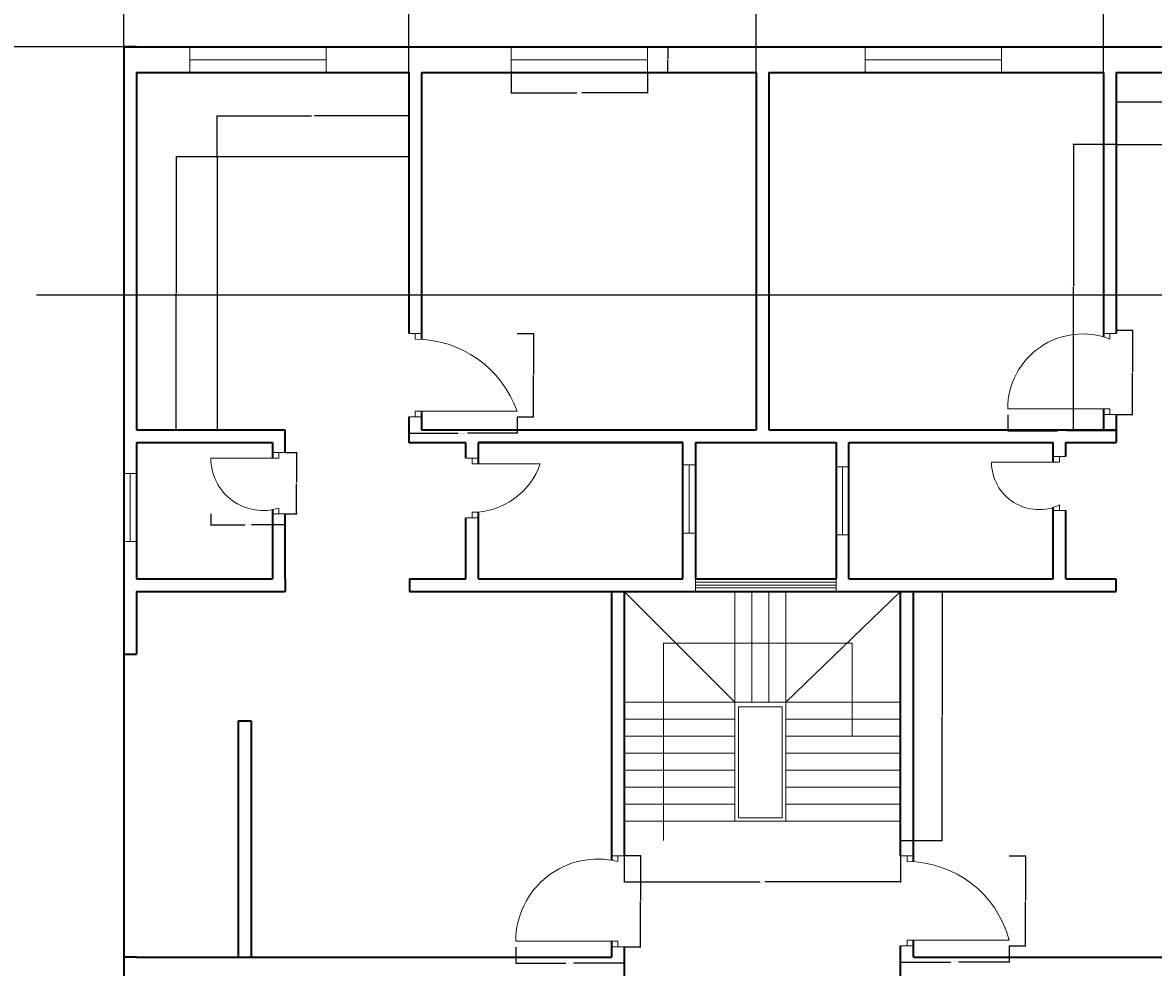
# Model space of a CAD drawing. Units: inches. Extents: x 2043 to 3387, y 1535 to 2797.
# Tile 5 of 7: x 2688 to 3087, y 2002 to 2335. Entities that reach past the tile are written whole.
import ezdxf

# ---------------------------------------------------------------- set-up
doc = ezdxf.new("R2010")
doc.units = ezdxf.units.IN
for name, color, linetype, lineweight in [('A-ANNO-DIMS', 2, 'Continuous', 18), ('A-ANNO-SYMB', 2, 'Continuous', 25), ('A-DOOR', 3, 'Continuous', 18), ('A-FLOR-FIXT', 9, 'Continuous', 25), ('A-FLOR-STRS', 2, 'Continuous', 18), ('A-GLAZ', 4, 'Continuous', 18), ('A-WALL', 7, 'Continuous', 35)]:
    doc.layers.add(name, color=color, linetype=linetype, lineweight=lineweight)
doc.styles.get("Standard").update_dxf_attribs({"font": 'arial.ttf'})
doc.dimstyles.get("Standard").update_dxf_attribs({"dimtxt": 0.18, "dimasz": 0.18, "dimexe": 0.18, "dimexo": 0.0625, "dimgap": 0.09, "dimtad": 0, "dimtih": 1, "dimtoh": 1, "dimdec": 4, "dimzin": 0, "dimdsep": 46, "dimtxsty": 'Standard', "dimcen": 0.09, "dimadec": 0, "dimazin": 0, "dimtfac": 1, "dimtdec": 4, "dimtofl": 0, "dimtmove": 0, "dimatfit": 3, "dimfxl": 1, "dimtolj": 1, "dimtzin": 0, "dimarcsym": 0})

# ---------------------------------------------------------------- blocks, each defined once
blk = doc.blocks.new('DOOR-24-WC-NW')
for p, q in [((21.75, 21.53), (26.25, 21.53)), ((26.25, 21.53), (24, 21.53)), ((24, 21.53), (24, 19.53)), ((24, 19.53), (0, 19.53)), ((24, 0), (24, 2)), ((26.25, 0), (21.75, 0)), ((21.75, 0), (24, 0))]:
    blk.add_line(p, q)
blk.add_arc((18.4, 19.53), 18.41, 180, 287.6967)
blk = doc.blocks.new('DOOR-36-BED-NW')
for p, q in [((0, 29.41), (4.5, 29.41)), ((4.5, 29.41), (2.25, 29.41)), ((2.25, 29.41), (2.25, 27.41)), ((4.5, 0), (0, 0)), ((0, 0), (2.25, 0)), ((2.25, 0), (2.25, 2)), ((2.25, 2), (38.25, 2))]:
    blk.add_line(p, q)
blk.add_arc((2.25, -10.79), 38.2, 19.5607, 90)
blk = doc.blocks.new('DOOR-36-BED-NE')
for p, q in [((33.75, 28.58), (38.25, 28.58)), ((38.25, 28.58), (36, 28.58)), ((36, 28.58), (36, 26.58)), ((36, 2), (0, 2)), ((38.25, 0), (33.75, 0)), ((33.75, 0), (36, 0)), ((36, 0), (36, 2))]:
    blk.add_line(p, q)
blk.add_arc((26.39, 2), 26.39, 68.6481, 180)
blk = doc.blocks.new('DOOR-24-BATH-NW')
for p, q in [((0, 21.1), (4.5, 21.1)), ((4.5, 21.1), (2.25, 21.1)), ((2.25, 21.1), (2.25, 19.1)), ((2.25, 19.1), (26.25, 19.1)), ((2.25, 0), (2.25, 2)), ((0, 0), (4.5, 0)), ((4.5, 0), (2.25, 0))]:
    blk.add_line(p, q)
blk.add_arc((2.25, 27.39), 25.39, 270, 340.9383)
blk = doc.blocks.new('DOOR-24-BATH-NE')
for p, q in [((24, 17.07), (0, 17.07)), ((26.25, 19.07), (21.75, 19.07)), ((21.75, 19.07), (24, 19.07)), ((24, 19.07), (24, 17.07)), ((24, 0), (24, 2)), ((21.75, 0), (26.25, 0)), ((26.25, 0), (24, 0))]:
    blk.add_line(p, q)
blk.add_arc((16.73, 17.07), 16.73, 180, 295.7467)
blk = doc.blocks.new('DOOR-36-ENTRY-NW')
for p, q in [((33.75, 32.08), (38.25, 32.08)), ((38.25, 32.08), (36, 32.08)), ((36, 32.08), (36, 30.08)), ((36, 2), (0, 2)), ((33.75, 0), (38.25, 0)), ((36, 0), (36, 2)), ((38.25, 0), (36, 0))]:
    blk.add_line(p, q)
blk.add_arc((28.95, 2), 28.95, 75.8996, 180)
blk = doc.blocks.new('DOOR-36-ENTRY-NE')
for p, q in [((0, 31.7), (3.27, 31.7)), ((4.5, 31.7), (2.28, 31.7)), ((2.28, 31.7), (2.28, 29.7)), ((3.27, 31.7), (4.5, 31.7)), ((0, 0), (4.5, 0)), ((4.5, 0), (0, 0)), ((0, 0), (2.25, 0)), ((2.25, 0), (2.25, 2)), ((2.25, 2), (38.25, 2))]:
    blk.add_line(p, q)
blk.add_arc((2.28, -7.5), 37.2, 14.7934, 90)
blk = doc.blocks.new('COUNTER-L-NW')
for p, q in [((67.52, 96.23), (0, 96.23)), ((0, 96.23), (0, 0))]:
    blk.add_line(p, q)
blk = doc.blocks.new('COUNTER-L-NE')
for p, q in [((0, 100.61), (68.19, 100.61)), ((68.19, 100.61), (68.19, 0))]:
    blk.add_line(p, q)
blk = doc.blocks.new('STAIR-U-RETURN')
for p, q in [((0, 87.81), (0, 48.81)), ((39, 48.81), (0, 87.81)), ((39, 48.81), (39, 87.81)), ((45, 48.81), (45, 87.81)), ((51, 48.81), (51, 87.81)), ((57, 48.81), (57, 87.81)), ((57, 48.81), (97.5, 87.81)), ((97.5, 87.81), (58.5, 87.81)), ((13.82, 0), (13.82, 69.54)), ((13.82, 69.54), (80.42, 69.54)), ((80.42, 69.54), (80.42, 36.81)), ((0, 48.81), (39, 48.81)), ((57, 48.81), (39, 48.81)), ((39, 48.81), (39, 48.81)), ((39, 48.81), (39, 6.81)), ((57, 48.81), (57, 6.81)), ((57, 48.81), (97.5, 48.81)), ((0, 42.81), (39, 42.81)), ((57, 42.81), (97.5, 42.81)), ((0, 36.81), (39, 36.81)), ((57, 36.81), (97.5, 36.81)), ((0, 30.81), (39, 30.81)), ((57, 30.81), (97.5, 30.81)), ((0, 24.81), (39, 24.81)), ((57, 24.81), (97.5, 24.81)), ((0, 18.81), (39, 18.81)), ((57, 18.81), (97.5, 18.81)), ((0, 12.81), (39, 12.81)), ((57, 12.81), (97.5, 12.81)), ((0, 6.81), (39, 6.81)), ((39, 6.81), (57, 6.81)), ((57, 6.81), (97.5, 6.81))]:
    blk.add_line(p, q)
blk.add_lwpolyline([(40.29, 47.17), (55.75, 47.17), (55.75, 8.03), (40.29, 8.03)], close=True)
blk = doc.blocks.new('WIN-48-PLAN')
for p, q in [((0, 9), (0, 0)), ((48, 4.5), (48, 9)), ((48, 9), (48, 0)), ((0, 0), (0, 4.5)), ((0, 4.5), (48, 4.5))]:
    blk.add_line(p, q)
blk = doc.blocks.new('WIN-48-N-JAMB')
for p, q in [((0, 9), (0, 0)), ((0, 0), (0, 9)), ((0, 9), (0, 4.5)), ((48, 4.5), (48, 9)), ((48, 9), (48, 0)), ((0, 4.5), (48, 4.5))]:
    blk.add_line(p, q)
blk = doc.blocks.new('VENT-24-W')
for p, q in [((0, 24), (4.5, 24)), ((4.5, 24), (0, 24)), ((0, 24), (0, 0)), ((2.25, 24), (2.25, 0)), ((0, 0), (4.5, 0))]:
    blk.add_line(p, q)
blk = doc.blocks.new('VENT-24-PLAN')
for p, q in [((0, 24), (4.5, 24)), ((4.5, 24), (2.25, 24)), ((2.25, 24), (2.25, 0)), ((2.25, 0), (0, 0)), ((0, 0), (4.5, 0))]:
    blk.add_line(p, q)
blk = doc.blocks.new('WIN-STAIR-DUCT')
for p, q in [((0, 4.5), (0, 0)), ((49.62, 4.5), (49.62, 0)), ((0, 2.25), (0, 3.25)), ((0, 3.25), (49.62, 3.25)), ((49.62, 2.25), (0, 2.25)), ((49.62, 1.25), (0, 1.25)), ((49.62, 3.25), (49.62, 2.25)), ((49.62, 2.25), (49.62, 2.25)), ((49.62, 2.25), (49.62, 1.25))]:
    blk.add_line(p, q)
blk = doc.blocks.new('*D41')
at = {"layer": 'A-ANNO-DIMS', "color": 0, "lineweight": -2, "transparency": 16777216}
for p, q in [((2860.38, 2317.31), (2860.38, 2310)), ((2908.38, 2317.31), (2908.38, 2310)), ((2860.56, 2310.18), (2883.48, 2310.18)), ((2908.2, 2310.18), (2885.28, 2310.18))]:
    blk.add_line(p, q, dxfattribs=at)
at = {"layer": 'A-ANNO-DIMS', "color": 0, "transparency": 16777216}
for points in [[(2860.56, 2310.21), (2860.56, 2310.15), (2860.38, 2310.18)], [(2908.2, 2310.21), (2908.2, 2310.15), (2908.38, 2310.18)]]:
    blk.add_solid(points, dxfattribs=at)
at = {"layer": 'Defpoints', "color": 0, "transparency": 16777216}
for p in [(2860.38, 2317.38), (2908.38, 2317.38), (2908.38, 2310.18)]:
    blk.add_point(p, dxfattribs=at)
at = {"layer": 'A-ANNO-DIMS', "color": 0, "transparency": 16777216, "insert": (2884.38, 2310.18), "char_height": 0.18, "attachment_point": 5}
blk.add_mtext('\\A1;JAMB 48 TYP.', dxfattribs=at)
blk = doc.blocks.new('*D42')
at = {"layer": 'A-ANNO-DIMS', "color": 0, "lineweight": -2, "transparency": 16777216}
for p, q in [((2908.45, 2326.38), (2915.76, 2326.38)), ((2915.58, 2326.2), (2915.58, 2322.06)), ((2915.58, 2317.56), (2915.58, 2321.7)), ((2908.45, 2317.38), (2915.76, 2317.38))]:
    blk.add_line(p, q, dxfattribs=at)
at = {"layer": 'A-ANNO-DIMS', "color": 0, "transparency": 16777216}
for points in [[(2915.55, 2326.2), (2915.61, 2326.2), (2915.58, 2326.38)], [(2915.55, 2317.56), (2915.61, 2317.56), (2915.58, 2317.38)]]:
    blk.add_solid(points, dxfattribs=at)
at = {"layer": 'Defpoints', "color": 0, "transparency": 16777216}
for p in [(2908.38, 2326.38), (2915.58, 2326.38), (2908.38, 2317.38)]:
    blk.add_point(p, dxfattribs=at)
at = {"layer": 'A-ANNO-DIMS', "color": 0, "transparency": 16777216, "insert": (2915.58, 2321.88), "char_height": 0.18, "attachment_point": 5}
blk.add_mtext('\\A1;9 TYP.', dxfattribs=at)
blk = doc.blocks.new('*D49')
at = {"layer": 'A-ANNO-DIMS', "color": 0, "lineweight": -2, "transparency": 16777216}
for p, q in [((2754.46, 2161.73), (2754.46, 2157.68)), ((2780.71, 2161.73), (2780.71, 2157.68)), ((2754.64, 2157.86), (2766.4, 2157.86)), ((2780.53, 2157.86), (2768.77, 2157.86))]:
    blk.add_line(p, q, dxfattribs=at)
at = {"layer": 'A-ANNO-DIMS', "color": 0, "transparency": 16777216}
for points in [[(2754.64, 2157.89), (2754.64, 2157.83), (2754.46, 2157.86)], [(2780.53, 2157.89), (2780.53, 2157.83), (2780.71, 2157.86)]]:
    blk.add_solid(points, dxfattribs=at)
at = {"layer": 'Defpoints', "color": 0, "transparency": 16777216}
for p in [(2754.46, 2161.79), (2780.71, 2161.79), (2780.71, 2157.86)]:
    blk.add_point(p, dxfattribs=at)
at = {"layer": 'A-ANNO-DIMS', "color": 0, "transparency": 16777216, "insert": (2767.58, 2157.86), "char_height": 0.18, "attachment_point": 5}
blk.add_mtext('\\A1;WC DOOR 26 TYP.', dxfattribs=at)
blk = doc.blocks.new('*D50')
at = {"layer": 'A-ANNO-DIMS', "color": 0, "lineweight": -2, "transparency": 16777216}
for p, q in [((2780.77, 2183.33), (2784.83, 2183.33)), ((2784.65, 2183.15), (2784.65, 2172.74)), ((2784.65, 2161.97), (2784.65, 2172.38)), ((2780.77, 2161.79), (2784.83, 2161.79))]:
    blk.add_line(p, q, dxfattribs=at)
at = {"layer": 'A-ANNO-DIMS', "color": 0, "transparency": 16777216}
for points in [[(2784.62, 2183.15), (2784.68, 2183.15), (2784.65, 2183.33)], [(2784.62, 2161.97), (2784.68, 2161.97), (2784.65, 2161.79)]]:
    blk.add_solid(points, dxfattribs=at)
at = {"layer": 'Defpoints', "color": 0, "transparency": 16777216}
for p in [(2780.71, 2183.33), (2784.65, 2183.33), (2780.71, 2161.79)]:
    blk.add_point(p, dxfattribs=at)
at = {"layer": 'A-ANNO-DIMS', "color": 0, "transparency": 16777216, "insert": (2784.65, 2172.56), "char_height": 0.18, "attachment_point": 5}
blk.add_mtext('\\A1;22 TYP.', dxfattribs=at)
blk = doc.blocks.new('*D65')
at = {"layer": 'A-ANNO-DIMS', "color": 0, "lineweight": -2, "transparency": 16777216}
for p, q in [((2861.96, 2008.98), (2861.96, 2003.13)), ((2900.21, 2008.98), (2900.21, 2003.13)), ((2862.14, 2003.31), (2879.69, 2003.31)), ((2900.03, 2003.31), (2882.48, 2003.31))]:
    blk.add_line(p, q, dxfattribs=at)
at = {"layer": 'A-ANNO-DIMS', "color": 0, "transparency": 16777216}
for points in [[(2862.14, 2003.34), (2862.14, 2003.28), (2861.96, 2003.31)], [(2900.03, 2003.34), (2900.03, 2003.28), (2900.21, 2003.31)]]:
    blk.add_solid(points, dxfattribs=at)
at = {"layer": 'Defpoints', "color": 0, "transparency": 16777216}
for p in [(2861.96, 2009.05), (2900.21, 2009.05), (2900.21, 2003.31)]:
    blk.add_point(p, dxfattribs=at)
at = {"layer": 'A-ANNO-DIMS', "color": 0, "transparency": 16777216, "insert": (2881.08, 2003.31), "char_height": 0.18, "attachment_point": 5}
blk.add_mtext('\\A1;ENTRY DOOR 38 TYP.', dxfattribs=at)
blk = doc.blocks.new('*D66')
at = {"layer": 'A-ANNO-DIMS', "color": 0, "lineweight": -2, "transparency": 16777216}
for p, q in [((2900.27, 2041.29), (2906.13, 2041.29)), ((2905.95, 2041.11), (2905.95, 2025.35)), ((2905.95, 2009.23), (2905.95, 2024.99)), ((2900.27, 2009.05), (2906.13, 2009.05))]:
    blk.add_line(p, q, dxfattribs=at)
at = {"layer": 'A-ANNO-DIMS', "color": 0, "transparency": 16777216}
for points in [[(2905.92, 2041.11), (2905.98, 2041.11), (2905.95, 2041.29)], [(2905.92, 2009.23), (2905.98, 2009.23), (2905.95, 2009.05)]]:
    blk.add_solid(points, dxfattribs=at)
at = {"layer": 'Defpoints', "color": 0, "transparency": 16777216}
for p in [(2900.21, 2041.29), (2905.95, 2041.29), (2900.21, 2009.05)]:
    blk.add_point(p, dxfattribs=at)
at = {"layer": 'A-ANNO-DIMS', "color": 0, "transparency": 16777216, "insert": (2905.95, 2025.17), "char_height": 0.18, "attachment_point": 5}
blk.add_mtext('\\A1;32 TYP.', dxfattribs=at)
blk = doc.blocks.new('*D67')
at = {"layer": 'A-ANNO-DIMS', "color": 0, "lineweight": -2, "transparency": 16777216}
for p, q in [((2997.71, 2009.36), (2997.71, 2003.5)), ((3035.96, 2009.36), (3035.96, 2003.5)), ((2997.89, 2003.68), (3015.44, 2003.68)), ((3035.78, 2003.68), (3018.23, 2003.68))]:
    blk.add_line(p, q, dxfattribs=at)
at = {"layer": 'A-ANNO-DIMS', "color": 0, "transparency": 16777216}
for points in [[(2997.89, 2003.71), (2997.89, 2003.65), (2997.71, 2003.68)], [(3035.78, 2003.71), (3035.78, 2003.65), (3035.96, 2003.68)]]:
    blk.add_solid(points, dxfattribs=at)
at = {"layer": 'Defpoints', "color": 0, "transparency": 16777216}
for p in [(2997.71, 2009.42), (3035.96, 2009.42), (3035.96, 2003.68)]:
    blk.add_point(p, dxfattribs=at)
at = {"layer": 'A-ANNO-DIMS', "color": 0, "transparency": 16777216, "insert": (3016.83, 2003.68), "char_height": 0.18, "attachment_point": 5}
blk.add_mtext('\\A1;ENTRY DOOR 38 TYP.', dxfattribs=at)
blk = doc.blocks.new('*D68')
at = {"layer": 'A-ANNO-DIMS', "color": 0, "lineweight": -2, "transparency": 16777216}
for p, q in [((3036.02, 2041.12), (3041.88, 2041.12)), ((3041.7, 2040.94), (3041.7, 2025.45)), ((3041.7, 2009.6), (3041.7, 2025.09)), ((3036.02, 2009.42), (3041.88, 2009.42))]:
    blk.add_line(p, q, dxfattribs=at)
at = {"layer": 'A-ANNO-DIMS', "color": 0, "transparency": 16777216}
for points in [[(3041.67, 2040.94), (3041.73, 2040.94), (3041.7, 2041.12)], [(3041.67, 2009.6), (3041.73, 2009.6), (3041.7, 2009.42)]]:
    blk.add_solid(points, dxfattribs=at)
at = {"layer": 'Defpoints', "color": 0, "transparency": 16777216}
for p in [(3035.96, 2041.12), (3041.7, 2041.12), (3035.96, 2009.42)]:
    blk.add_point(p, dxfattribs=at)
at = {"layer": 'A-ANNO-DIMS', "color": 0, "transparency": 16777216, "insert": (3041.7, 2025.27), "char_height": 0.18, "attachment_point": 5}
blk.add_mtext('\\A1;32 TYP.', dxfattribs=at)
blk = doc.blocks.new('*D73')
at = {"layer": 'A-ANNO-DIMS', "color": 0, "lineweight": -2, "transparency": 16777216}
for p, q in [((2824.21, 2195.88), (2824.21, 2190.03)), ((2862.46, 2195.88), (2862.46, 2190.03)), ((2824.39, 2190.21), (2841.71, 2190.21)), ((2862.28, 2190.21), (2844.95, 2190.21))]:
    blk.add_line(p, q, dxfattribs=at)
at = {"layer": 'A-ANNO-DIMS', "color": 0, "transparency": 16777216}
for points in [[(2824.39, 2190.24), (2824.39, 2190.18), (2824.21, 2190.21)], [(2862.28, 2190.24), (2862.28, 2190.18), (2862.46, 2190.21)]]:
    blk.add_solid(points, dxfattribs=at)
at = {"layer": 'Defpoints', "color": 0, "transparency": 16777216}
for p in [(2824.21, 2195.94), (2862.46, 2195.94), (2862.46, 2190.21)]:
    blk.add_point(p, dxfattribs=at)
at = {"layer": 'A-ANNO-DIMS', "color": 0, "transparency": 16777216, "insert": (2843.33, 2190.21), "char_height": 0.18, "attachment_point": 5}
blk.add_mtext('\\A1;BEDROOM DOOR 38 TYP.', dxfattribs=at)
blk = doc.blocks.new('*D74')
at = {"layer": 'A-ANNO-DIMS', "color": 0, "lineweight": -2, "transparency": 16777216}
for p, q in [((2862.52, 2225.36), (2868.38, 2225.36)), ((2868.2, 2225.18), (2868.2, 2210.83)), ((2868.2, 2196.12), (2868.2, 2210.47)), ((2862.52, 2195.94), (2868.38, 2195.94))]:
    blk.add_line(p, q, dxfattribs=at)
at = {"layer": 'A-ANNO-DIMS', "color": 0, "transparency": 16777216}
for points in [[(2868.17, 2225.18), (2868.23, 2225.18), (2868.2, 2225.36)], [(2868.17, 2196.12), (2868.23, 2196.12), (2868.2, 2195.94)]]:
    blk.add_solid(points, dxfattribs=at)
at = {"layer": 'Defpoints', "color": 0, "transparency": 16777216}
for p in [(2862.46, 2225.36), (2868.2, 2225.36), (2862.46, 2195.94)]:
    blk.add_point(p, dxfattribs=at)
at = {"layer": 'A-ANNO-DIMS', "color": 0, "transparency": 16777216, "insert": (2868.2, 2210.65), "char_height": 0.18, "attachment_point": 5}
blk.add_mtext('\\A1;29 TYP.', dxfattribs=at)
blk = doc.blocks.new('*D75')
at = {"layer": 'A-ANNO-DIMS', "color": 0, "lineweight": -2, "transparency": 16777216}
for p, q in [((3035.46, 2196.71), (3035.46, 2190.86)), ((3073.71, 2196.71), (3073.71, 2190.86)), ((3035.64, 2191.04), (3052.96, 2191.04)), ((3073.53, 2191.04), (3056.2, 2191.04))]:
    blk.add_line(p, q, dxfattribs=at)
at = {"layer": 'A-ANNO-DIMS', "color": 0, "transparency": 16777216}
for points in [[(3035.64, 2191.07), (3035.64, 2191.01), (3035.46, 2191.04)], [(3073.53, 2191.07), (3073.53, 2191.01), (3073.71, 2191.04)]]:
    blk.add_solid(points, dxfattribs=at)
at = {"layer": 'Defpoints', "color": 0, "transparency": 16777216}
for p in [(3035.46, 2196.78), (3073.71, 2196.78), (3073.71, 2191.04)]:
    blk.add_point(p, dxfattribs=at)
at = {"layer": 'A-ANNO-DIMS', "color": 0, "transparency": 16777216, "insert": (3054.58, 2191.04), "char_height": 0.18, "attachment_point": 5}
blk.add_mtext('\\A1;BEDROOM DOOR 38 TYP.', dxfattribs=at)
blk = doc.blocks.new('*D76')
at = {"layer": 'A-ANNO-DIMS', "color": 0, "lineweight": -2, "transparency": 16777216}
for p, q in [((3073.77, 2226.53), (3079.63, 2226.53)), ((3079.45, 2226.35), (3079.45, 2211.84)), ((3079.45, 2196.96), (3079.45, 2211.47)), ((3073.77, 2196.78), (3079.63, 2196.78))]:
    blk.add_line(p, q, dxfattribs=at)
at = {"layer": 'A-ANNO-DIMS', "color": 0, "transparency": 16777216}
for points in [[(3079.42, 2226.35), (3079.48, 2226.35), (3079.45, 2226.53)], [(3079.42, 2196.96), (3079.48, 2196.96), (3079.45, 2196.78)]]:
    blk.add_solid(points, dxfattribs=at)
at = {"layer": 'Defpoints', "color": 0, "transparency": 16777216}
for p in [(3073.71, 2226.53), (3079.45, 2226.53), (3073.71, 2196.78)]:
    blk.add_point(p, dxfattribs=at)
at = {"layer": 'A-ANNO-DIMS', "color": 0, "transparency": 16777216, "insert": (3079.45, 2211.65), "char_height": 0.18, "attachment_point": 5}
blk.add_mtext('\\A1;30 TYP.', dxfattribs=at)
blk = doc.blocks.new('*D81')
at = {"layer": 'A-ANNO-DIMS', "color": 0, "lineweight": -2, "transparency": 16777216}
for p, q in [((2756.63, 2287.61), (2742.08, 2287.61)), ((2742.26, 2287.43), (2742.26, 2239.68)), ((2742.26, 2191.56), (2742.26, 2239.31)), ((2756.63, 2191.38), (2742.08, 2191.38))]:
    blk.add_line(p, q, dxfattribs=at)
at = {"layer": 'A-ANNO-DIMS', "color": 0, "transparency": 16777216}
for points in [[(2742.23, 2287.43), (2742.29, 2287.43), (2742.26, 2287.61)], [(2742.23, 2191.56), (2742.29, 2191.56), (2742.26, 2191.38)]]:
    blk.add_solid(points, dxfattribs=at)
at = {"layer": 'Defpoints', "color": 0, "transparency": 16777216}
for p in [(2742.26, 2287.61), (2756.69, 2287.61), (2756.69, 2191.38)]:
    blk.add_point(p, dxfattribs=at)
at = {"layer": 'A-ANNO-DIMS', "color": 0, "transparency": 16777216, "insert": (2742.26, 2239.49), "char_height": 0.18, "attachment_point": 5}
blk.add_mtext('\\A1;COUNTER 96 TYP.', dxfattribs=at)
blk = doc.blocks.new('*D82')
at = {"layer": 'A-ANNO-DIMS', "color": 0, "lineweight": -2, "transparency": 16777216}
for p, q in [((2756.69, 2287.67), (2756.69, 2302.22)), ((2756.87, 2302.04), (2789.92, 2302.04)), ((2824.03, 2302.04), (2790.98, 2302.04)), ((2824.21, 2287.67), (2824.21, 2302.22))]:
    blk.add_line(p, q, dxfattribs=at)
at = {"layer": 'A-ANNO-DIMS', "color": 0, "transparency": 16777216}
for points in [[(2756.87, 2302.07), (2756.87, 2302.01), (2756.69, 2302.04)], [(2824.03, 2302.07), (2824.03, 2302.01), (2824.21, 2302.04)]]:
    blk.add_solid(points, dxfattribs=at)
at = {"layer": 'Defpoints', "color": 0, "transparency": 16777216}
for p in [(2824.21, 2302.04), (2756.69, 2287.61), (2824.21, 2287.61)]:
    blk.add_point(p, dxfattribs=at)
at = {"layer": 'A-ANNO-DIMS', "color": 0, "transparency": 16777216, "insert": (2790.45, 2302.04), "char_height": 0.18, "attachment_point": 5}
blk.add_mtext('\\A1;68 TYP.', dxfattribs=at)
blk = doc.blocks.new('*D83')
at = {"layer": 'A-ANNO-DIMS', "color": 0, "lineweight": -2, "transparency": 16777216}
for p, q in [((3073.65, 2291.99), (3058.44, 2291.99)), ((3058.62, 2291.81), (3058.62, 2241.87)), ((3058.62, 2191.56), (3058.62, 2241.5)), ((3073.65, 2191.38), (3058.44, 2191.38))]:
    blk.add_line(p, q, dxfattribs=at)
at = {"layer": 'A-ANNO-DIMS', "color": 0, "transparency": 16777216}
for points in [[(3058.59, 2291.81), (3058.65, 2291.81), (3058.62, 2291.99)], [(3058.59, 2191.56), (3058.65, 2191.56), (3058.62, 2191.38)]]:
    blk.add_solid(points, dxfattribs=at)
at = {"layer": 'Defpoints', "color": 0, "transparency": 16777216}
for p in [(3058.62, 2291.99), (3073.71, 2291.99), (3073.71, 2191.38)]:
    blk.add_point(p, dxfattribs=at)
at = {"layer": 'A-ANNO-DIMS', "color": 0, "transparency": 16777216, "insert": (3058.62, 2241.68), "char_height": 0.18, "attachment_point": 5}
blk.add_mtext('\\A1;COUNTER 101 TYP.', dxfattribs=at)
blk = doc.blocks.new('*D84')
at = {"layer": 'A-ANNO-DIMS', "color": 0, "lineweight": -2, "transparency": 16777216}
for p, q in [((3073.71, 2292.05), (3073.71, 2307.26)), ((3073.89, 2307.08), (3107.27, 2307.08)), ((3141.72, 2307.08), (3108.33, 2307.08)), ((3141.9, 2292.05), (3141.9, 2307.26))]:
    blk.add_line(p, q, dxfattribs=at)
at = {"layer": 'A-ANNO-DIMS', "color": 0, "transparency": 16777216}
for points in [[(3073.89, 2307.11), (3073.89, 2307.05), (3073.71, 2307.08)], [(3141.72, 2307.11), (3141.72, 2307.05), (3141.9, 2307.08)]]:
    blk.add_solid(points, dxfattribs=at)
at = {"layer": 'Defpoints', "color": 0, "transparency": 16777216}
for p in [(3141.9, 2307.08), (3073.71, 2291.99), (3141.9, 2291.99)]:
    blk.add_point(p, dxfattribs=at)
at = {"layer": 'A-ANNO-DIMS', "color": 0, "transparency": 16777216, "insert": (3107.8, 2307.08), "char_height": 0.18, "attachment_point": 5}
blk.add_mtext('\\A1;68 TYP.', dxfattribs=at)
blk = doc.blocks.new('*D89')
at = {"layer": 'A-ANNO-DIMS', "color": 0, "lineweight": -2, "transparency": 16777216}
for p, q in [((2900.21, 2046.51), (2900.21, 2031.76)), ((2997.71, 2046.51), (2997.71, 2031.76)), ((2900.39, 2031.94), (2948.03, 2031.94)), ((2997.53, 2031.94), (2949.89, 2031.94))]:
    blk.add_line(p, q, dxfattribs=at)
at = {"layer": 'A-ANNO-DIMS', "color": 0, "transparency": 16777216}
for points in [[(2900.39, 2031.97), (2900.39, 2031.91), (2900.21, 2031.94)], [(2997.53, 2031.97), (2997.53, 2031.91), (2997.71, 2031.94)]]:
    blk.add_solid(points, dxfattribs=at)
at = {"layer": 'Defpoints', "color": 0, "transparency": 16777216}
for p in [(2900.21, 2046.57), (2997.71, 2046.57), (2997.71, 2031.94)]:
    blk.add_point(p, dxfattribs=at)
at = {"layer": 'A-ANNO-DIMS', "color": 0, "transparency": 16777216, "insert": (2948.96, 2031.94), "char_height": 0.18, "attachment_point": 5}
blk.add_mtext('\\A1;STAIR 98 TYP.', dxfattribs=at)
blk = doc.blocks.new('*D90')
at = {"layer": 'A-ANNO-DIMS', "color": 0, "lineweight": -2, "transparency": 16777216}
for p, q in [((2997.77, 2134.38), (3012.51, 2134.38)), ((3012.33, 2134.2), (3012.33, 2090.65)), ((3012.33, 2046.75), (3012.33, 2090.29)), ((2997.77, 2046.57), (3012.51, 2046.57))]:
    blk.add_line(p, q, dxfattribs=at)
at = {"layer": 'A-ANNO-DIMS', "color": 0, "transparency": 16777216}
for points in [[(3012.3, 2134.2), (3012.36, 2134.2), (3012.33, 2134.38)], [(3012.3, 2046.75), (3012.36, 2046.75), (3012.33, 2046.57)]]:
    blk.add_solid(points, dxfattribs=at)
at = {"layer": 'Defpoints', "color": 0, "transparency": 16777216}
for p in [(2997.71, 2134.38), (3012.33, 2134.38), (2997.71, 2046.57)]:
    blk.add_point(p, dxfattribs=at)
at = {"layer": 'A-ANNO-DIMS', "color": 0, "transparency": 16777216, "insert": (3012.33, 2090.47), "char_height": 0.18, "attachment_point": 5}
blk.add_mtext('\\A1;88 TYP.', dxfattribs=at)
blk = doc.blocks.new('*D106')
at = {"layer": 'A-ANNO-DIMS', "color": 0, "lineweight": -2, "transparency": 16777216}
for p, q in [((2723.65, 2326.38), (2660.13, 2326.38)), ((2660.31, 2326.2), (2660.31, 2006.31)), ((2660.31, 1686.06), (2660.31, 2005.95)), ((2723.65, 1685.88), (2660.13, 1685.88))]:
    blk.add_line(p, q, dxfattribs=at)
at = {"layer": 'A-ANNO-DIMS', "color": 0, "transparency": 16777216}
for points in [[(2660.28, 2326.2), (2660.34, 2326.2), (2660.31, 2326.38)], [(2660.28, 1686.06), (2660.34, 1686.06), (2660.31, 1685.88)]]:
    blk.add_solid(points, dxfattribs=at)
at = {"layer": 'Defpoints', "color": 0, "transparency": 16777216}
for p in [(2660.31, 2326.38), (2723.71, 2326.38), (2723.71, 1685.88)]:
    blk.add_point(p, dxfattribs=at)
at = {"layer": 'A-ANNO-DIMS', "color": 0, "transparency": 16777216, "insert": (2660.31, 2006.13), "char_height": 0.18, "attachment_point": 5}
blk.add_mtext('\\A1;640.5', dxfattribs=at)
blk = doc.blocks.new('*D107')
at = {"layer": 'A-ANNO-DIMS', "color": 0, "lineweight": -2, "transparency": 16777216}
for p, q in [((2723.71, 2326.44), (2723.71, 2359.26)), ((2723.89, 2359.08), (2773.57, 2359.08)), ((2824.03, 2359.08), (2774.34, 2359.08)), ((2824.21, 2317.44), (2824.21, 2359.26))]:
    blk.add_line(p, q, dxfattribs=at)
at = {"layer": 'A-ANNO-DIMS', "color": 0, "transparency": 16777216}
for points in [[(2723.89, 2359.11), (2723.89, 2359.05), (2723.71, 2359.08)], [(2824.03, 2359.11), (2824.03, 2359.05), (2824.21, 2359.08)]]:
    blk.add_solid(points, dxfattribs=at)
at = {"layer": 'Defpoints', "color": 0, "transparency": 16777216}
for p in [(2824.21, 2359.08), (2723.71, 2326.38), (2824.21, 2317.38)]:
    blk.add_point(p, dxfattribs=at)
at = {"layer": 'A-ANNO-DIMS', "color": 0, "transparency": 16777216, "insert": (2773.96, 2359.08), "char_height": 0.18, "attachment_point": 5}
blk.add_mtext('\\A1;100.5', dxfattribs=at)
blk = doc.blocks.new('*D108')
at = {"layer": 'A-ANNO-DIMS', "color": 0, "lineweight": -2, "transparency": 16777216}
for p, q in [((2824.21, 2317.44), (2824.21, 2359.26)), ((2824.39, 2359.08), (2885.07, 2359.08)), ((2946.53, 2359.08), (2885.84, 2359.08)), ((2946.71, 2317.44), (2946.71, 2359.26))]:
    blk.add_line(p, q, dxfattribs=at)
at = {"layer": 'A-ANNO-DIMS', "color": 0, "transparency": 16777216}
for points in [[(2824.39, 2359.11), (2824.39, 2359.05), (2824.21, 2359.08)], [(2946.53, 2359.11), (2946.53, 2359.05), (2946.71, 2359.08)]]:
    blk.add_solid(points, dxfattribs=at)
at = {"layer": 'Defpoints', "color": 0, "transparency": 16777216}
for p in [(2946.71, 2359.08), (2824.21, 2317.38), (2946.71, 2317.38)]:
    blk.add_point(p, dxfattribs=at)
at = {"layer": 'A-ANNO-DIMS', "color": 0, "transparency": 16777216, "insert": (2885.46, 2359.08), "char_height": 0.18, "attachment_point": 5}
blk.add_mtext('\\A1;122.5', dxfattribs=at)
blk = doc.blocks.new('*D109')
at = {"layer": 'A-ANNO-DIMS', "color": 0, "lineweight": -2, "transparency": 16777216}
for p, q in [((2946.71, 2317.44), (2946.71, 2359.26)), ((2946.89, 2359.08), (3007.57, 2359.08)), ((3069.03, 2359.08), (3008.34, 2359.08)), ((3069.21, 2317.44), (3069.21, 2359.26))]:
    blk.add_line(p, q, dxfattribs=at)
at = {"layer": 'A-ANNO-DIMS', "color": 0, "transparency": 16777216}
for points in [[(2946.89, 2359.11), (2946.89, 2359.05), (2946.71, 2359.08)], [(3069.03, 2359.11), (3069.03, 2359.05), (3069.21, 2359.08)]]:
    blk.add_solid(points, dxfattribs=at)
at = {"layer": 'Defpoints', "color": 0, "transparency": 16777216}
for p in [(3069.21, 2359.08), (2946.71, 2317.38), (3069.21, 2317.38)]:
    blk.add_point(p, dxfattribs=at)
at = {"layer": 'A-ANNO-DIMS', "color": 0, "transparency": 16777216, "insert": (3007.96, 2359.08), "char_height": 0.18, "attachment_point": 5}
blk.add_mtext('\\A1;122.5', dxfattribs=at)
blk = doc.blocks.new('*D110')
at = {"layer": 'A-ANNO-DIMS', "color": 0, "lineweight": -2, "transparency": 16777216}
for p, q in [((3069.21, 2317.44), (3069.21, 2359.26)), ((3069.39, 2359.08), (3121.43, 2359.08)), ((3174.03, 2359.08), (3121.99, 2359.08)), ((3174.21, 2326.44), (3174.21, 2359.26))]:
    blk.add_line(p, q, dxfattribs=at)
at = {"layer": 'A-ANNO-DIMS', "color": 0, "transparency": 16777216}
for points in [[(3069.39, 2359.11), (3069.39, 2359.05), (3069.21, 2359.08)], [(3174.03, 2359.11), (3174.03, 2359.05), (3174.21, 2359.08)]]:
    blk.add_solid(points, dxfattribs=at)
at = {"layer": 'Defpoints', "color": 0, "transparency": 16777216}
for p in [(3174.21, 2359.08), (3174.21, 2326.38), (3069.21, 2317.38)]:
    blk.add_point(p, dxfattribs=at)
at = {"layer": 'A-ANNO-DIMS', "color": 0, "transparency": 16777216, "insert": (3121.71, 2359.08), "char_height": 0.18, "attachment_point": 5}
blk.add_mtext('\\A1;105', dxfattribs=at)

msp = doc.modelspace()

# ---------------------------------------------------------------- linework, layer by layer
at = {"layer": 'A-ANNO-SYMB'}
msp.add_line((2693.0063, 2238.9239), (3223.9712, 2238.9239), dxfattribs=at)
at = {"layer": 'A-WALL'}
for p, q in [((2723.7086, 2326.3769), (3174.2086, 2326.3769)), ((2728.2086, 2326.3769), (2723.7086, 2326.3769)), ((2723.7086, 2326.3769), (2723.7086, 1734.4589)), ((2728.2086, 2317.3769), (2824.2086, 2317.3769)), ((2728.2086, 2317.3769), (2728.2086, 2191.3769)), ((2824.2086, 2317.3769), (2824.2086, 2225.357)), ((2828.7086, 2317.3769), (2946.7086, 2317.3769)), ((2828.7086, 2317.3769), (2828.7086, 2223.2907)), ((2946.7086, 2317.3769), (2946.7086, 2191.3769)), ((2951.2086, 2317.3769), (3069.2086, 2317.3769)), ((2951.2086, 2317.3769), (2951.2086, 2191.3769)), ((3069.2086, 2317.3769), (3069.2086, 2224.1217)), ((3073.7086, 2317.3769), (3169.7086, 2317.3769)), ((3073.7086, 2317.3769), (3073.7086, 2225.357)), ((2828.7086, 2197.9433), (2828.7086, 2191.3769)), ((3069.2086, 2198.7773), (3069.2086, 2191.3769)), ((2824.2086, 2195.9433), (2824.2086, 2186.8769)), ((3073.7086, 2196.7773), (3073.7086, 2186.8769)), ((2728.2086, 2191.3769), (2780.7086, 2191.3769)), ((2780.7086, 2183.3291), (2780.7086, 2191.3769)), ((2828.7086, 2191.3769), (2946.7086, 2191.3769)), ((2951.2086, 2191.3769), (3069.2086, 2191.3769)), ((2728.2086, 2186.8769), (2776.2086, 2186.8769)), ((2728.2086, 2186.8769), (2728.2086, 2138.8769)), ((2728.2086, 2186.8769), (2776.2086, 2186.8769)), ((2776.2086, 2186.8769), (2776.2086, 2181.3291)), ((2824.2086, 2186.8769), (2844.3641, 2186.8769)), ((2824.2086, 2186.8769), (2844.3641, 2186.8769)), ((2844.3641, 2181.3932), (2844.3641, 2186.8769)), ((2848.8641, 2186.8769), (2920.8641, 2186.8769)), ((2848.8641, 2186.8769), (2896.2086, 2186.8769)), ((2848.8641, 2179.3932), (2848.8641, 2186.8769)), ((2920.8641, 2186.8769), (2848.8641, 2186.8769)), ((2920.8641, 2138.8769), (2920.8641, 2186.8769)), ((2925.3641, 2186.8769), (2974.9865, 2186.8769)), ((2925.3641, 2186.8769), (2925.3641, 2138.8769)), ((2974.9865, 2186.8769), (2974.9865, 2138.8769)), ((2979.4865, 2186.8769), (3051.4865, 2186.8769)), ((2979.4865, 2138.8769), (2979.4865, 2186.8769)), ((3051.4865, 2179.9477), (3051.4865, 2186.8769)), ((3055.9865, 2186.8769), (3073.7086, 2186.8769)), ((3055.9865, 2181.9477), (3055.9865, 2186.8769)), ((2776.2086, 2163.2304), (2776.2086, 2138.8769)), ((2780.7086, 2138.8769), (2780.7086, 2161.7948)), ((2848.8641, 2138.8769), (2848.8641, 2162.3935)), ((3051.4865, 2138.8769), (3051.4865, 2163.9861)), ((3055.9865, 2138.8769), (3055.9865, 2162.8769)), ((2844.3641, 2138.8769), (2844.3641, 2160.2936)), ((2728.2086, 2138.8769), (2776.2086, 2138.8769)), ((2780.7086, 2138.8769), (2780.7086, 2134.3769)), ((2824.5414, 2138.8769), (2844.3641, 2138.8769)), ((2824.5414, 2138.8769), (2824.5414, 2134.3769)), ((2848.8641, 2138.8769), (2920.8641, 2138.8769)), ((2925.3641, 2138.8769), (2974.9865, 2138.8769)), ((2979.4865, 2138.8769), (3051.4865, 2138.8769)), ((3055.9865, 2138.8769), (3073.6281, 2138.8769)), ((3073.6281, 2138.8769), (3073.6281, 2134.3769)), ((2728.2086, 2134.3769), (2780.7086, 2134.3769)), ((2728.2086, 2134.3769), (2728.2086, 2112.2282)), ((2824.5414, 2134.3769), (2828.7086, 2134.3769)), ((2828.7086, 2134.3769), (2951.2086, 2134.3769)), ((2895.7086, 2134.3769), (2895.7086, 2039.5927)), ((2900.2086, 2134.3769), (2900.2086, 2041.1216)), ((2951.2086, 2134.3769), (3073.7086, 2134.3769)), ((2997.7086, 2041.1216), (2997.7086, 2134.3769)), ((3002.2086, 2039.0555), (3002.2086, 2134.3769)), ((2723.7086, 2112.2282), (2728.2086, 2112.2282)), ((2764.2086, 2005.3769), (2764.2086, 2088.7241)), ((2764.2086, 2088.7241), (2768.7086, 2088.7241)), ((2768.7086, 2088.7241), (2768.7086, 2005.3769)), ((2895.7086, 2011.0461), (2895.7086, 2005.3769)), ((3002.2086, 2005.3769), (3002.2086, 2011.4195)), ((2900.2086, 2009.0461), (2900.2086, 1994.0737)), ((2997.7086, 1994.6872), (2997.7086, 2009.4195)), ((2728.2086, 2005.3769), (2723.7086, 2005.3769)), ((2728.2086, 2005.3769), (2895.7086, 2005.3769)), ((2728.2086, 2005.3769), (2764.2086, 2005.3769)), ((3002.2086, 2005.3769), (3174.2086, 2005.3769))]:
    msp.add_line(p, q, dxfattribs=at)

# ---------------------------------------------------------------- block references
at = {"layer": 'A-DOOR'}
for name, p in [('DOOR-36-BED-NW', (2824.209, 2195.943)), ('DOOR-36-BED-NE', (3035.459, 2196.777)), ('DOOR-24-WC-NW', (2754.459, 2161.795)), ('DOOR-24-BATH-NW', (2844.364, 2160.294)), ('DOOR-24-BATH-NE', (3029.737, 2162.877)), ('DOOR-36-ENTRY-NW', (2861.959, 2009.046)), ('DOOR-36-ENTRY-NE', (2997.709, 2009.419))]:
    msp.add_blockref(name, p, dxfattribs=at)
at = {"layer": 'A-FLOR-FIXT'}
for name, p in [('COUNTER-L-NE', (3073.709, 2191.377)), ('COUNTER-L-NW', (2756.693, 2191.377))]:
    msp.add_blockref(name, p, dxfattribs=at)
at = {"layer": 'A-FLOR-STRS'}
msp.add_blockref('STAIR-U-RETURN', (2900.209, 2046.569), dxfattribs=at)
at = {"layer": 'A-GLAZ'}
for name, p in [('WIN-48-PLAN', (2747.069, 2317.377)), ('WIN-48-N-JAMB', (2860.383, 2317.377)), ('WIN-48-PLAN', (2985.2127, 2317.377)), ('VENT-24-W', (2723.709, 2151.93)), ('WIN-STAIR-DUCT', (2925.364, 2134.377))]:
    msp.add_blockref(name, p, dxfattribs=at)
at = {"layer": 'A-GLAZ', "rotation": 180}
for p in [(2925.3637, 2178.9772), (2979.4861, 2178.2836)]:
    msp.add_blockref('VENT-24-PLAN', p, dxfattribs=at)

# ---------------------------------------------------------------- dimensions: what is measured, and where the dimension line sits
at = {"layer": 'A-ANNO-DIMS'}
for base, p1, p2, override, picture, middle in [((2824.2086, 2359.0769), (2723.7086, 2326.3769), (2824.2086, 2317.3769), {"dimdec": 1, "dimlfac": 1, "dimrnd": 0, "dimzin": 0, "dimdsep": 46, "dimlunit": 2}, '*D107', (2773.9586, 2359.0769)), ((2946.7086, 2359.0769), (2824.2086, 2317.3769), (2946.7086, 2317.3769), {"dimdec": 1, "dimlfac": 1, "dimrnd": 0, "dimzin": 0, "dimdsep": 46, "dimlunit": 2}, '*D108', (2885.4586, 2359.0769)), ((3069.2086, 2359.0769), (2946.7086, 2317.3769), (3069.2086, 2317.3769), {"dimdec": 1, "dimlfac": 1, "dimrnd": 0, "dimzin": 0, "dimdsep": 46, "dimlunit": 2}, '*D109', (3007.9586, 2359.0769)), ((3174.2086, 2359.0769), (3069.2086, 2317.3769), (3174.2086, 2326.3769), {"dimdec": 0, "dimlfac": 1, "dimrnd": 0, "dimzin": 0, "dimdsep": 46, "dimlunit": 2}, '*D110', (3121.7086, 2359.0769))]:
    dim = msp.add_linear_dim(base=base, p1=p1, p2=p2, dimstyle='Standard', override=override, dxfattribs=at)
    dim.commit()
    dim.dimension.update_dxf_attribs({"geometry": picture, "text_midpoint": middle})
dim = msp.add_linear_dim(base=(2660.3063, 2326.3769), p1=(2723.7086, 1685.8769), p2=(2723.7086, 2326.3769), angle=90, dimstyle='Standard', override={"dimdec": 1, "dimlfac": 1, "dimrnd": 0, "dimzin": 0, "dimdsep": 46, "dimlunit": 2}, dxfattribs=at)
dim.commit()
dim.dimension.update_dxf_attribs({"geometry": '*D106', "text_midpoint": (2660.3063, 2006.1269)})
for base, p1, p2, text, picture, middle in [((2915.5829, 2326.3769), (2908.3829, 2317.3769), (2908.3829, 2326.3769), '<> TYP.', '*D42', (2915.5829, 2321.8769)), ((3058.6169, 2291.9886), (3073.7086, 2191.3769), (3073.7086, 2291.9886), 'COUNTER <> TYP.', '*D83', (3058.6169, 2241.6828)), ((2742.2586, 2287.607), (2756.6931, 2191.3769), (2756.6931, 2287.607), 'COUNTER <> TYP.', '*D81', (2742.2586, 2239.492)), ((2868.1961, 2225.357), (2862.4586, 2195.9433), (2862.4586, 2225.357), '<> TYP.', '*D74', (2868.1961, 2210.6502)), ((3079.4461, 2226.5321), (3073.7086, 2196.7773), (3073.7086, 2226.5321), '<> TYP.', '*D76', (3079.4461, 2211.6547)), ((2784.6461, 2183.3291), (2780.7086, 2161.7948), (2780.7086, 2183.3291), '<> TYP.', '*D50', (2784.6461, 2172.562)), ((3012.3336, 2134.3769), (2997.7086, 2046.5688), (2997.7086, 2134.3769), '<> TYP.', '*D90', (3012.3336, 2090.4729)), ((2905.9461, 2041.2946), (2900.2086, 2009.0461), (2900.2086, 2041.2946), '<> TYP.', '*D66', (2905.9461, 2025.1704)), ((3041.6961, 2041.1216), (3035.9586, 2009.4195), (3035.9586, 2041.1216), '<> TYP.', '*D68', (3041.6961, 2025.2706))]:
    dim = msp.add_linear_dim(base=base, p1=p1, p2=p2, angle=90, text=text, dimstyle='Standard', override={"dimdec": 0, "dimlfac": 1, "dimrnd": 0, "dimzin": 0, "dimdsep": 46, "dimlunit": 2}, dxfattribs=at)
    dim.commit()
    dim.dimension.update_dxf_attribs({"geometry": picture, "text_midpoint": middle})
for base, p1, p2, text, picture, middle in [((2908.3829, 2310.1769), (2860.3829, 2317.3769), (2908.3829, 2317.3769), 'JAMB <> TYP.', '*D41', (2884.3829, 2310.1769)), ((3141.8962, 2307.0803), (3073.7086, 2291.9886), (3141.8962, 2291.9886), '<> TYP.', '*D84', (3107.8024, 2307.0803)), ((2824.2086, 2302.0415), (2756.6931, 2287.607), (2824.2086, 2287.607), '<> TYP.', '*D82', (2790.4508, 2302.0415)), ((2862.4586, 2190.2058), (2824.2086, 2195.9433), (2862.4586, 2195.9433), 'BEDROOM DOOR <> TYP.', '*D73', (2843.3336, 2190.2058)), ((3073.7086, 2191.0398), (3035.4586, 2196.7773), (3073.7086, 2196.7773), 'BEDROOM DOOR <> TYP.', '*D75', (3054.5836, 2191.0398)), ((2780.7086, 2157.8573), (2754.4586, 2161.7948), (2780.7086, 2161.7948), 'WC DOOR <> TYP.', '*D49', (2767.5836, 2157.8573)), ((2997.7086057422, 2031.9438100763), (2900.2086057422, 2046.5688100763), (2997.7086057422, 2046.5688100763), 'STAIR <> TYP.', '*D89', (2948.9586057422, 2031.9438100763)), ((2900.2086, 2003.3086), (2861.9586, 2009.0461), (2900.2086, 2009.0461), 'ENTRY DOOR <> TYP.', '*D65', (2881.0836, 2003.3086)), ((3035.9586, 2003.682), (2997.7086, 2009.4195), (3035.9586, 2009.4195), 'ENTRY DOOR <> TYP.', '*D67', (3016.8336, 2003.682))]:
    dim = msp.add_linear_dim(base=base, p1=p1, p2=p2, text=text, dimstyle='Standard', override={"dimdec": 0, "dimlfac": 1, "dimrnd": 0, "dimzin": 0, "dimdsep": 46, "dimlunit": 2}, dxfattribs=at)
    dim.commit()
    dim.dimension.update_dxf_attribs({"geometry": picture, "text_midpoint": middle})

doc.saveas('drawing.dxf')
